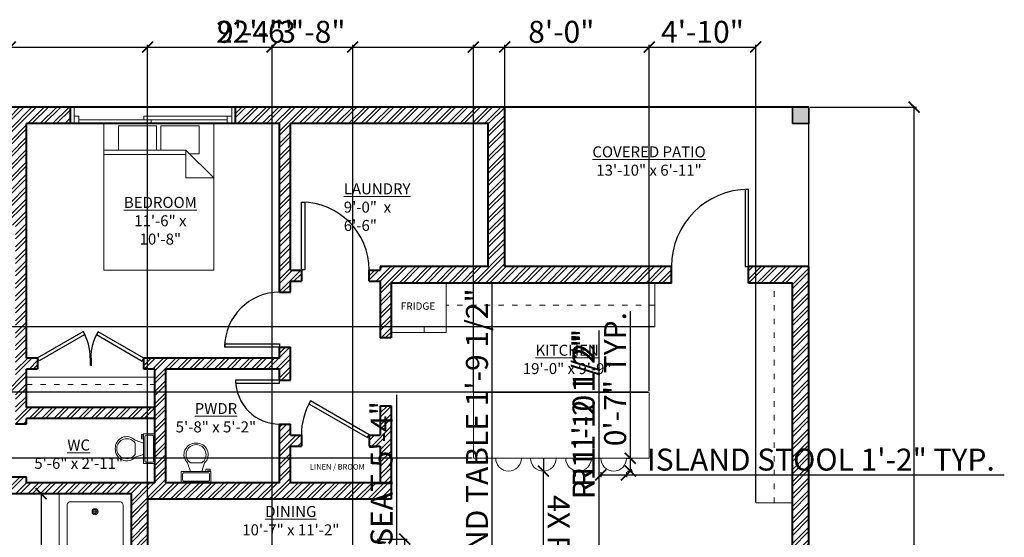
# Model space of a CAD drawing. Units: inches. Extents: x 982 to 1904, y 735 to 1463.
# Tile 7 of 7: x 1301 to 1838, y 1160 to 1443. Entities that reach past the tile are written whole.
import ezdxf

# ---------------------------------------------------------------- set-up
doc = ezdxf.new("R2010")
doc.units = ezdxf.units.IN
doc.linetypes.add('ACAD_ISO03W100', pattern=[30, 12, -18])
for name, color, linetype, lineweight in [('A-ANNO-TEXT', 7, 'Continuous', 18), ('A-AREA-IDEN', 7, 'Continuous', 18), ('A-COLS', 7, 'Continuous', 35), ('A-EQPM', 8, 'Continuous', 18), ('A-FLOR', 7, 'Continuous', 25), ('A-FLOR-CASE', 8, 'Continuous', 20), ('A-FLOR-CASE-HIDN', 8, 'ACAD_ISO03W100', 13), ('A-FLOR-FIXT', 70, 'Continuous', 20), ('Dimensions', 9, 'Continuous', 18), ('Doors', 130, 'Continuous', 25), ('Furniture', 31, 'Continuous', 18), ('Wall Hatch', 23, 'Continuous', 13), ('Walls', 151, 'Continuous', 40), ('Windows', 111, 'Continuous', 18)]:
    doc.layers.add(name, color=color, linetype=linetype, lineweight=lineweight)
doc.layers.add('A-COLS-PATT', color=251, linetype='Continuous', lineweight=13, true_color=0x636466)
doc.styles.get("Standard").update_dxf_attribs({"font": 'arial.ttf'})
doc.dimstyles.new('ISO-25', dxfattribs={"dimtxt": 12, "dimasz": 6, "dimexe": 1.25, "dimexo": 0.625, "dimtad": 1, "dimlunit": 3, "dimtxsty": 'Standard', "dimblk": 'ARCHTICK', "dimcen": 2.5, "dimadec": 0, "dimazin": 0, "dimtfac": 1, "dimtmove": 0, "dimatfit": 3, "dimfxl": 1, "dimarcsym": 0})

# ---------------------------------------------------------------- blocks, each defined once
blk = doc.blocks.new('*U7')
for p, q in [((9.5, -6), (9.5, -2)), ((-10, -8.5), (-8, -8.5)), ((-10, -9.5), (-10, -8.5)), ((-7, -9.5), (-10, -9.5)), ((-8, -8.5), (-8, -8)), ((-7, -8), (-7, -9.5)), ((-4, -8), (-6, -14)), ((4, -8), (6, -14)), ((4, -14), (-4, -14))]:
    blk.add_line(p, q)
blk.add_lwpolyline([(10.5, -8), (10.5, 0), (-10.5, 0), (-10.5, -8)], close=True)
for points in [[(-9.5, -2), (-9.5, -6)], [(8.5, -1), (-8.5, -1)], [(-8.5, -7), (8.5, -7)]]:
    blk.add_lwpolyline(points)
for centre, radius, start, end in [((-8.625, -1.875), 0.8839, 81.8699, 188.1301), ((-8.625, -6.125), 0.8839, 171.869898, 278.1301), ((8.625, -1.875), 0.8839, 351.8699, 98.1301), ((8.625, -6.125), 0.8839, 261.8699, 8.1301), ((-0.4772, -19.9188), 8.0953, 133.01722, 273.38), ((0.0374, -19.8731), 7.127, 124.50543, 269.7), ((-0.0373, -19.8731), 7.127, 270.3, 55.4946), ((0.4773, -19.9188), 8.0953, 266.62, 46.9828)]:
    blk.add_arc(centre, radius, start, end)
blk = doc.blocks.new('*U11')
for p, q in [((0, 0), (0, -100)), ((900, 0), (900, -100))]:
    blk.add_line(p, q)
blk.add_lwpolyline([(0, 0), (0, 900), (43.75, 900), (43.75, 0)], close=True)
blk.add_arc((0, 0), 900, 0, 90)
blk = doc.blocks.new('*U12')
for p, q in [((0, 0), (0, -100)), ((-1000, 0), (-1000, -100))]:
    blk.add_line(p, q)
blk.add_lwpolyline([(0, 0), (0, 1000), (-43.75, 1000), (-43.75, 0)], close=True)
blk.add_arc((0, 0), 1000, 90, 180)
blk = doc.blocks.new('*U13')
for p, q in [((0, 0), (0, -100)), ((-900, 0), (-900, -100))]:
    blk.add_line(p, q)
blk.add_lwpolyline([(0, 0), (-779, 450), (-801, 412), (-22, -38)], close=True)
blk.add_arc((0, 0), 900, 150, 180)
blk = doc.blocks.new('*U14')
for p, q in [((0, 0), (0, -100)), ((750, 0), (750, -100))]:
    blk.add_line(p, q)
blk.add_lwpolyline([(0, 0), (0, 750), (43.75, 750), (43.75, 0)], close=True)
blk.add_arc((0, 0), 750, 0, 90)
blk = doc.blocks.new('*U15')
for p, q in [((-600, 0), (-600, -100)), ((0, 0), (0, -100))]:
    blk.add_line(p, q)
blk.add_lwpolyline([(0, 0), (0, 600), (-43.75, 600), (-43.75, 0)], close=True)
blk.add_arc((0, 0), 600, 90, 180)
blk = doc.blocks.new('Bed - Queen')
for p, q in [((0, -80.00003), (0, 0)), ((0, 0), (59.99999, 0)), ((59.99999, 0), (59.99999, -80.00003)), ((7.99999, -1.2), (28.79998, -1.2)), ((7.99999, -14.4), (7.99999, -1.2)), ((28.79998, -1.2), (28.79998, -14.4)), ((31.19999, -1.2), (51.99999, -1.2)), ((31.19999, -14.4), (31.19999, -1.2)), ((51.99999, -1.2), (51.99999, -16.4)), ((0, -14.4), (44.8, -14.4)), ((59.99999, -29.6), (44.8, -14.4)), ((44.8, -14.4), (44.8, -29.6)), ((44.8, -16.8), (0, -16.8)), ((51.99999, -16.4), (46.79936, -16.4)), ((44.8, -29.6), (59.99999, -29.6)), ((59.99999, -80.00003), (0, -80.00003))]:
    blk.add_line(p, q)
blk = doc.blocks.new('*U17')
for p, q in [((0, 0), (0, -100)), ((700, 0), (700, -100))]:
    blk.add_line(p, q)
blk.add_lwpolyline([(0, 0), (606, 350), (628, 312), (22, -38)], close=True)
blk.add_arc((0, 0), 700, 0, 30)
blk = doc.blocks.new('Bath Tub - 26 x 60 in.')
for p, q in [((8, -18), (10, -18)), ((9, -17), (9, -19))]:
    blk.add_line(p, q)
blk.add_lwpolyline([(0, -36), (0, 0), (60, 0), (60, -36)], close=True)
for points in [[(6, -4), (42, -4)], [(4, -30), (4, -6)], [(42, -32), (6, -32)]]:
    blk.add_lwpolyline(points)
for radius in [1.5, 1]:
    blk.add_circle((9, -18), radius)
for centre, radius, start, end in [((5.75, -5.75), 1.77, 81.8699, 188.1301), ((42, -18), 14, 270, 90), ((5.75, -30.25), 1.77, 171.8699, 278.1301)]:
    blk.add_arc(centre, radius, start, end)
blk = doc.blocks.new('_ArchTick')
at = {"color": 0, "linetype": 'ByBlock', "const_width": 0.15}
blk.add_lwpolyline([(-0.5, -0.5), (0.5, 0.5)], dxfattribs=at)
blk = doc.blocks.new('*D23')
at = {"layer": 'Defpoints', "color": 0, "transparency": 16777216}
for p in [(1731.5, 1394.99), (1788.92, 1394.99), (1732.75, 812.49)]:
    blk.add_point(p, dxfattribs=at)
at = {"layer": 'Dimensions', "color": 0, "lineweight": -2, "transparency": 16777216}
for p, q in [((1732.12, 1394.99), (1790.17, 1394.99)), ((1788.92, 812.49), (1788.92, 1394.99)), ((1733.37, 812.49), (1790.17, 812.49))]:
    blk.add_line(p, q, dxfattribs=at)
at = {"layer": 'Dimensions', "color": 0, "lineweight": -2, "transparency": 16777216, "xscale": 6, "yscale": 6, "zscale": 6}
for p, rotation in [((1788.92, 1394.99), 90), ((1788.92, 812.49), 270)]:
    blk.add_blockref('_ArchTick', p, dxfattribs=dict(at, rotation=rotation))
at = {"layer": 'Dimensions', "color": 0, "transparency": 16777216, "insert": (1782.16, 1103.74), "char_height": 12, "attachment_point": 5, "rotation": 90}
blk.add_mtext('48\'-6.5"', dxfattribs=at)
blk = doc.blocks.new('ISLAND-STOOL-14')
blk.add_arc((7, 7), 7, 180, 0)
blk = doc.blocks.new('*D30')
at = {"layer": 'Defpoints', "color": 0, "transparency": 16777216}
for p in [(1617.95, 1196.33), (1631.95, 1196.33), (1631.95, 1194.23)]:
    blk.add_point(p, dxfattribs=at)
at = {"layer": 'Dimensions', "color": 0, "lineweight": -2, "transparency": 16777216}
for p, q in [((1617.95, 1195.7), (1617.95, 1192.98)), ((1617.95, 1194.23), (1631.95, 1194.23)), ((1631.95, 1195.7), (1631.95, 1192.98)), ((1631.95, 1194.23), (1838.17, 1194.23))]:
    blk.add_line(p, q, dxfattribs=at)
at = {"layer": 'Dimensions', "color": 0, "lineweight": -2, "transparency": 16777216, "xscale": 6, "yscale": 6, "zscale": 6, "rotation": 180}
blk.add_blockref('_ArchTick', (1617.95, 1194.23), dxfattribs=at)
at = {"layer": 'Dimensions', "color": 0, "lineweight": -2, "transparency": 16777216, "xscale": 6, "yscale": 6, "zscale": 6}
blk.add_blockref('_ArchTick', (1631.95, 1194.23), dxfattribs=at)
at = {"layer": 'Dimensions', "color": 0, "transparency": 16777216, "insert": (1738.06, 1201.06), "char_height": 12, "attachment_point": 5}
blk.add_mtext('ISLAND STOOL 1\'-2" TYP.', dxfattribs=at)
blk = doc.blocks.new('*D31')
at = {"layer": 'Defpoints', "color": 0, "transparency": 16777216}
for p in [(1631.95, 1203.33), (1634.05, 1203.33), (1631.95, 1196.33)]:
    blk.add_point(p, dxfattribs=at)
at = {"layer": 'Dimensions', "color": 0, "lineweight": -2, "transparency": 16777216}
for p, q in [((1634.05, 1203.33), (1634.05, 1283.72)), ((1632.57, 1203.33), (1635.3, 1203.33)), ((1634.05, 1196.33), (1634.05, 1203.33)), ((1632.57, 1196.33), (1635.3, 1196.33))]:
    blk.add_line(p, q, dxfattribs=at)
at = {"layer": 'Dimensions', "color": 0, "lineweight": -2, "transparency": 16777216, "xscale": 6, "yscale": 6, "zscale": 6}
for p, rotation in [((1634.05, 1203.33), 90), ((1634.05, 1196.33), 270)]:
    blk.add_blockref('_ArchTick', p, dxfattribs=dict(at, rotation=rotation))
at = {"layer": 'Dimensions', "color": 0, "transparency": 16777216, "insert": (1627.29, 1246.53), "char_height": 12, "attachment_point": 5, "rotation": 90}
blk.add_mtext('0\'-7" TYP.', dxfattribs=at)
blk = doc.blocks.new('*D41')
at = {"layer": 'Defpoints', "color": 0, "transparency": 16777216}
for p in [(1495.17, 1159.23), (1510.97, 1159.23), (1495.17, 1095.57)]:
    blk.add_point(p, dxfattribs=at)
at = {"layer": 'Dimensions', "color": 0, "lineweight": -2, "transparency": 16777216}
for p, q in [((1495.79, 1159.23), (1512.22, 1159.23)), ((1510.97, 1095.57), (1510.97, 1159.23)), ((1495.79, 1095.57), (1512.22, 1095.57))]:
    blk.add_line(p, q, dxfattribs=at)
at = {"layer": 'Dimensions', "color": 0, "lineweight": -2, "transparency": 16777216, "xscale": 6, "yscale": 6, "zscale": 6}
for p, rotation in [((1510.97, 1159.23), 90), ((1510.97, 1095.57), 270)]:
    blk.add_blockref('_ArchTick', p, dxfattribs=dict(at, rotation=rotation))
at = {"layer": 'Dimensions', "color": 0, "transparency": 16777216, "insert": (1504.14, 1127.4), "char_height": 12, "attachment_point": 5, "rotation": 90}
blk.add_mtext('5\'-3 1/2"', dxfattribs=at)
blk = doc.blocks.new('*D44')
at = {"layer": 'Defpoints', "color": 0, "transparency": 16777216}
for p in [(1506.61, 1106.1), (1516.2, 1106.1), (1516.2, 1042.21)]:
    blk.add_point(p, dxfattribs=at)
at = {"layer": 'Dimensions', "color": 0, "lineweight": -2, "transparency": 16777216}
for p, q in [((1506.61, 1106.1), (1506.61, 1237.89)), ((1515.57, 1106.1), (1505.36, 1106.1)), ((1506.61, 1042.21), (1506.61, 1106.1)), ((1515.57, 1042.21), (1505.36, 1042.21))]:
    blk.add_line(p, q, dxfattribs=at)
at = {"layer": 'Dimensions', "color": 0, "lineweight": -2, "transparency": 16777216, "xscale": 6, "yscale": 6, "zscale": 6}
for p, rotation in [((1506.61, 1106.1), 90), ((1506.61, 1042.21), 270)]:
    blk.add_blockref('_ArchTick', p, dxfattribs=dict(at, rotation=rotation))
at = {"layer": 'Dimensions', "color": 0, "transparency": 16777216, "insert": (1499.78, 1175), "char_height": 12, "attachment_point": 5, "rotation": 90}
blk.add_mtext('LOVESEAT 5\'-4"', dxfattribs=at)
blk = doc.blocks.new('*D48')
at = {"layer": 'Defpoints', "color": 0, "transparency": 16777216}
for p in [(1555.46, 1134.17), (1558.68, 1134.17), (1555.46, 1112.72)]:
    blk.add_point(p, dxfattribs=at)
at = {"layer": 'Dimensions', "color": 0, "lineweight": -2, "transparency": 16777216}
for p, q in [((1558.68, 1134.17), (1558.68, 1298.47)), ((1556.09, 1134.17), (1559.93, 1134.17)), ((1558.68, 1112.72), (1558.68, 1134.17)), ((1556.09, 1112.72), (1559.93, 1112.72))]:
    blk.add_line(p, q, dxfattribs=at)
at = {"layer": 'Dimensions', "color": 0, "lineweight": -2, "transparency": 16777216, "xscale": 6, "yscale": 6, "zscale": 6}
for p, rotation in [((1558.68, 1134.17), 90), ((1558.68, 1112.72), 270)]:
    blk.add_blockref('_ArchTick', p, dxfattribs=dict(at, rotation=rotation))
at = {"layer": 'Dimensions', "color": 0, "transparency": 16777216, "insert": (1551.85, 1219.32), "char_height": 12, "attachment_point": 5, "rotation": 90}
blk.add_mtext('END TABLE 1\'-9 1/2"', dxfattribs=at)
blk = doc.blocks.new('*D52')
at = {"layer": 'Defpoints', "color": 0, "transparency": 16777216}
for p in [(1322.2, 1183.99), (1312.37, 1118.49), (1322.2, 1118.49)]:
    blk.add_point(p, dxfattribs=at)
at = {"layer": 'Dimensions', "color": 0, "lineweight": -2, "transparency": 16777216}
for p, q in [((1321.57, 1183.99), (1311.12, 1183.99)), ((1312.37, 1183.99), (1312.37, 1118.49)), ((1321.57, 1118.49), (1311.12, 1118.49)), ((1312.37, 1118.49), (1312.37, 969.02))]:
    blk.add_line(p, q, dxfattribs=at)
at = {"layer": 'Dimensions', "color": 0, "lineweight": -2, "transparency": 16777216, "xscale": 6, "yscale": 6, "zscale": 6}
for p, rotation in [((1312.37, 1183.99), 90), ((1312.37, 1118.49), 270)]:
    blk.add_blockref('_ArchTick', p, dxfattribs=dict(at, rotation=rotation))
at = {"layer": 'Dimensions', "color": 0, "transparency": 16777216, "insert": (1305.54, 1040.75), "char_height": 12, "attachment_point": 5, "rotation": 90}
blk.add_mtext('BATHTUB 5\'-5 1/2"', dxfattribs=at)
blk = doc.blocks.new('*D60')
at = {"layer": 'Defpoints', "color": 0, "transparency": 16777216}
for p in [(1565.5, 1427.79), (1295.5, 1394.99), (1565.5, 1394.99)]:
    blk.add_point(p, dxfattribs=at)
at = {"layer": 'Dimensions', "color": 0, "lineweight": -2, "transparency": 16777216}
for p, q in [((1295.5, 1395.62), (1295.5, 1429.04)), ((1295.5, 1427.79), (1565.5, 1427.79)), ((1565.5, 1395.62), (1565.5, 1429.04))]:
    blk.add_line(p, q, dxfattribs=at)
at = {"layer": 'Dimensions', "color": 0, "lineweight": -2, "transparency": 16777216, "xscale": 6, "yscale": 6, "zscale": 6, "rotation": 180}
blk.add_blockref('_ArchTick', (1295.5, 1427.79), dxfattribs=at)
at = {"layer": 'Dimensions', "color": 0, "lineweight": -2, "transparency": 16777216, "xscale": 6, "yscale": 6, "zscale": 6}
blk.add_blockref('_ArchTick', (1565.5, 1427.79), dxfattribs=at)
at = {"layer": 'Dimensions', "color": 0, "transparency": 16777216, "insert": (1430.5, 1434.54), "char_height": 12, "attachment_point": 5}
blk.add_mtext('22\'-6"', dxfattribs=at)
blk = doc.blocks.new('*D64')
at = {"layer": 'Defpoints', "color": 0, "transparency": 16777216}
for p in [(1482.5, 1427.79), (1370.5, 841.99), (1482.5, 841.99)]:
    blk.add_point(p, dxfattribs=at)
at = {"layer": 'Dimensions', "color": 0, "lineweight": -2, "transparency": 16777216}
for p, q in [((1370.5, 842.62), (1370.5, 1429.04)), ((1370.5, 1427.79), (1482.5, 1427.79)), ((1482.5, 842.62), (1482.5, 1429.04))]:
    blk.add_line(p, q, dxfattribs=at)
at = {"layer": 'Dimensions', "color": 0, "lineweight": -2, "transparency": 16777216, "xscale": 6, "yscale": 6, "zscale": 6, "rotation": 180}
blk.add_blockref('_ArchTick', (1370.5, 1427.79), dxfattribs=at)
at = {"layer": 'Dimensions', "color": 0, "lineweight": -2, "transparency": 16777216, "xscale": 6, "yscale": 6, "zscale": 6}
blk.add_blockref('_ArchTick', (1482.5, 1427.79), dxfattribs=at)
at = {"layer": 'Dimensions', "color": 0, "transparency": 16777216, "insert": (1426.5, 1434.54), "char_height": 12, "attachment_point": 5}
blk.add_mtext('9\'-4"', dxfattribs=at)
blk = doc.blocks.new('*D66')
at = {"layer": 'Defpoints', "color": 0, "transparency": 16777216}
for p in [(1482.5, 1427.79), (1438.5, 1043.01), (1482.5, 1043.03)]:
    blk.add_point(p, dxfattribs=at)
at = {"layer": 'Dimensions', "color": 0, "lineweight": -2, "transparency": 16777216}
for p, q in [((1438.5, 1043.64), (1438.5, 1429.04)), ((1438.5, 1427.79), (1482.5, 1427.79)), ((1482.5, 1043.65), (1482.5, 1429.04))]:
    blk.add_line(p, q, dxfattribs=at)
at = {"layer": 'Dimensions', "color": 0, "lineweight": -2, "transparency": 16777216, "xscale": 6, "yscale": 6, "zscale": 6, "rotation": 180}
blk.add_blockref('_ArchTick', (1438.5, 1427.79), dxfattribs=at)
at = {"layer": 'Dimensions', "color": 0, "lineweight": -2, "transparency": 16777216, "xscale": 6, "yscale": 6, "zscale": 6}
blk.add_blockref('_ArchTick', (1482.5, 1427.79), dxfattribs=at)
at = {"layer": 'Dimensions', "color": 0, "transparency": 16777216, "insert": (1460.5, 1434.55), "char_height": 12, "attachment_point": 5}
blk.add_mtext('3\'-8"', dxfattribs=at)
blk = doc.blocks.new('*D67')
at = {"layer": 'Defpoints', "color": 0, "transparency": 16777216}
for p in [(1644.35, 1427.79), (1548.35, 1239.33), (1644.35, 1239.33)]:
    blk.add_point(p, dxfattribs=at)
at = {"layer": 'Dimensions', "color": 0, "lineweight": -2, "transparency": 16777216}
for p, q in [((1548.35, 1239.95), (1548.35, 1429.04)), ((1548.35, 1427.79), (1644.35, 1427.79)), ((1644.35, 1239.95), (1644.35, 1429.04))]:
    blk.add_line(p, q, dxfattribs=at)
at = {"layer": 'Dimensions', "color": 0, "lineweight": -2, "transparency": 16777216, "xscale": 6, "yscale": 6, "zscale": 6, "rotation": 180}
blk.add_blockref('_ArchTick', (1548.35, 1427.79), dxfattribs=at)
at = {"layer": 'Dimensions', "color": 0, "lineweight": -2, "transparency": 16777216, "xscale": 6, "yscale": 6, "zscale": 6}
blk.add_blockref('_ArchTick', (1644.35, 1427.79), dxfattribs=at)
at = {"layer": 'Dimensions', "color": 0, "transparency": 16777216, "insert": (1596.35, 1434.54), "char_height": 12, "attachment_point": 5}
blk.add_mtext('8\'-0"', dxfattribs=at)
blk = doc.blocks.new('*D68')
at = {"layer": 'Defpoints', "color": 0, "transparency": 16777216}
for p in [(1548.35, 1239.33), (1123.7, 1203.33), (1548.35, 1203.33)]:
    blk.add_point(p, dxfattribs=at)
at = {"layer": 'Dimensions', "color": 0, "lineweight": -2, "transparency": 16777216}
for p, q in [((1547.73, 1239.33), (1122.45, 1239.33)), ((1123.7, 1239.33), (1123.7, 1203.33)), ((1547.73, 1203.33), (1122.45, 1203.33))]:
    blk.add_line(p, q, dxfattribs=at)
at = {"layer": 'Dimensions', "color": 0, "lineweight": -2, "transparency": 16777216, "xscale": 6, "yscale": 6, "zscale": 6}
for p, rotation in [((1123.7, 1239.33), 90), ((1123.7, 1203.33), 270)]:
    blk.add_blockref('_ArchTick', p, dxfattribs=dict(at, rotation=rotation))
at = {"layer": 'Dimensions', "color": 0, "transparency": 16777216, "insert": (1116.94, 1221.33), "char_height": 12, "attachment_point": 5, "rotation": 90}
blk.add_mtext('3\'-0"', dxfattribs=at)
blk = doc.blocks.new('*D69')
at = {"layer": 'Defpoints', "color": 0, "transparency": 16777216}
for p in [(1123.7, 1274.99), (1647.5, 1274.99), (1644.35, 1239.33)]:
    blk.add_point(p, dxfattribs=at)
at = {"layer": 'Dimensions', "color": 0, "lineweight": -2, "transparency": 16777216}
for p, q in [((1123.7, 1274.99), (1123.7, 1351.63)), ((1646.87, 1274.99), (1122.45, 1274.99)), ((1123.7, 1239.33), (1123.7, 1274.99)), ((1643.73, 1239.33), (1122.45, 1239.33))]:
    blk.add_line(p, q, dxfattribs=at)
at = {"layer": 'Dimensions', "color": 0, "lineweight": -2, "transparency": 16777216, "xscale": 6, "yscale": 6, "zscale": 6}
for p, rotation in [((1123.7, 1274.99), 90), ((1123.7, 1239.33), 270)]:
    blk.add_blockref('_ArchTick', p, dxfattribs=dict(at, rotation=rotation))
at = {"layer": 'Dimensions', "color": 0, "transparency": 16777216, "insert": (1116.87, 1316.31), "char_height": 12, "attachment_point": 5, "rotation": 90}
blk.add_mtext('2\'-11 1/2"', dxfattribs=at)
blk = doc.blocks.new('*D70')
at = {"layer": 'Defpoints', "color": 0, "transparency": 16777216}
for p in [(1702.5, 1427.79), (1644.35, 1239.33), (1702.5, 1178.99)]:
    blk.add_point(p, dxfattribs=at)
at = {"layer": 'Dimensions', "color": 0, "lineweight": -2, "transparency": 16777216}
for p, q in [((1644.35, 1239.95), (1644.35, 1429.04)), ((1644.35, 1427.79), (1702.5, 1427.79)), ((1702.5, 1179.62), (1702.5, 1429.04))]:
    blk.add_line(p, q, dxfattribs=at)
at = {"layer": 'Dimensions', "color": 0, "lineweight": -2, "transparency": 16777216, "xscale": 6, "yscale": 6, "zscale": 6, "rotation": 180}
blk.add_blockref('_ArchTick', (1644.35, 1427.79), dxfattribs=at)
at = {"layer": 'Dimensions', "color": 0, "lineweight": -2, "transparency": 16777216, "xscale": 6, "yscale": 6, "zscale": 6}
blk.add_blockref('_ArchTick', (1702.5, 1427.79), dxfattribs=at)
at = {"layer": 'Dimensions', "color": 0, "transparency": 16777216, "insert": (1673.42, 1434.54), "char_height": 12, "attachment_point": 5}
blk.add_mtext('4\'-10"', dxfattribs=at)
blk = doc.blocks.new('*D73')
at = {"layer": 'Defpoints', "color": 0, "transparency": 16777216}
for p in [(1616.91, 1141.97), (1616.91, 999.48)]:
    blk.add_point(p, dxfattribs=at)
at = {"layer": 'Dimensions', "color": 0, "lineweight": -2, "transparency": 16777216}
for p in [(1616.91, 1273.09), (1616.91, 999.48)]:
    blk.add_line(p, (1616.91, 1141.97), dxfattribs=at)
at = {"layer": 'Dimensions', "color": 0, "lineweight": -2, "transparency": 16777216, "xscale": 6, "yscale": 6, "zscale": 6, "rotation": 269.9998576619989}
blk.add_blockref('_ArchTick', (1616.91, 1141.97), dxfattribs=at)
at = {"layer": 'Dimensions', "color": 0, "transparency": 16777216, "insert": (1610.08, 1227.47), "char_height": 12, "attachment_point": 5, "rotation": 89.9999}
blk.add_mtext('R11\'-10 1/2"', dxfattribs=at)
blk = doc.blocks.new('*D74')
at = {"layer": 'Defpoints', "color": 0, "transparency": 16777216}
for p in [(1616.91, 1149.03), (1616.91, 1014.7)]:
    blk.add_point(p, dxfattribs=at)
at = {"layer": 'Dimensions', "color": 0, "lineweight": -2, "transparency": 16777216}
for p in [(1616.91, 1270.59), (1616.91, 1014.7)]:
    blk.add_line(p, (1616.91, 1149.03), dxfattribs=at)
at = {"layer": 'Dimensions', "color": 0, "lineweight": -2, "transparency": 16777216, "xscale": 6, "yscale": 6, "zscale": 6, "rotation": 269.9998536992126}
blk.add_blockref('_ArchTick', (1616.91, 1149.03), dxfattribs=at)
at = {"layer": 'Dimensions', "color": 0, "transparency": 16777216, "insert": (1610.08, 1229.63), "char_height": 12, "attachment_point": 5, "rotation": 89.9999}
blk.add_mtext('R11\'-2 1/2"', dxfattribs=at)
blk = doc.blocks.new('*D79')
at = {"layer": 'Defpoints', "color": 0, "transparency": 16777216}
for p in [(1586.55, 1203.33), (1586.55, 1196.33)]:
    blk.add_point(p, dxfattribs=at)
at = {"layer": 'Dimensions', "color": 0, "lineweight": -2, "transparency": 16777216}
for p in [(1586.55, 1203.33), (1586.55, 1113.43)]:
    blk.add_line(p, (1586.55, 1196.33), dxfattribs=at)
at = {"layer": 'Dimensions', "color": 0, "lineweight": -2, "transparency": 16777216, "xscale": 6, "yscale": 6, "zscale": 6, "rotation": 90.00372422566393}
blk.add_blockref('_ArchTick', (1586.55, 1196.33), dxfattribs=at)
at = {"layer": 'Dimensions', "color": 0, "transparency": 16777216, "insert": (1593.3, 1148.88), "char_height": 12, "attachment_point": 5, "rotation": 270.0037}
blk.add_mtext('4X R0\'-7"', dxfattribs=at)

msp = doc.modelspace()

# ---------------------------------------------------------------- hatches: boundary and pattern name
at = {"layer": 'A-COLS-PATT'}
h = msp.add_hatch(color=256, dxfattribs=at)
h.dxf.hatch_style = 1
h.paths.add_polyline_path([(1731.496, 1394.991), (1722.496, 1394.991), (1722.496, 1385.991), (1731.496, 1385.991)])
h.paths.add_polyline_path([(1725.019, 843.656), (1721.019, 843.656), (1721.019, 837.656), (1725.019, 837.656)])
h.paths.add_polyline_path([(1734.019, 843.656), (1730.019, 843.656), (1730.019, 837.656), (1734.019, 837.656)])
h.paths.add_polyline_path([(1483.18, 791.991), (1479.18, 791.991), (1479.18, 785.991), (1483.18, 785.991)])
h.paths.add_polyline_path([(1492.18, 791.991), (1488.18, 791.991), (1488.18, 785.991), (1492.18, 785.991)])
h.paths.add_polyline_path([(1364.813, 791.991), (1360.813, 791.991), (1360.813, 785.991), (1364.813, 785.991)])
h.paths.add_polyline_path([(1373.813, 791.991), (1369.813, 791.991), (1369.813, 785.991), (1373.813, 785.991)])
at = {"layer": 'Wall Hatch'}
h = msp.add_hatch(dxfattribs=at)
h.set_pattern_fill('ANSI32', color=256, scale=0.5)
h.paths.add_polyline_path([(1165.496, 1065.991), (1271.496, 1065.991), (1271.496, 1071.991), (1218.496, 1071.991), (1218.496, 1238.491), (1262.496, 1238.491), (1262.496, 1244.491), (1218.496, 1244.491), (1218.496, 1330.491), (1298.496, 1330.491), (1298.496, 1244.491), (1292.496, 1244.491), (1292.496, 1238.491), (1298.496, 1238.491), (1298.496, 1221.991), (1304.496, 1221.991), (1304.496, 1224.991), (1374.496, 1224.991), (1374.496, 1230.991), (1304.496, 1230.991), (1304.496, 1251.991), (1310.496, 1251.991), (1310.496, 1257.991), (1304.496, 1257.991), (1304.496, 1385.991), (1328.496, 1385.991), (1328.496, 1394.991), (1295.496, 1394.991), (1295.496, 1339.491), (1209.496, 1339.491), (1209.496, 1071.991), (1156.496, 1071.991), (1156.496, 893.991), (1171.496, 893.991), (1171.496, 902.991), (1165.496, 902.991)])
h.paths.add_polyline_path([(1273.996, 877.991), (1267.996, 877.991), (1267.996, 902.991), (1252.996, 902.991), (1252.996, 893.991), (1258.996, 893.991), (1258.996, 868.991), (1273.996, 868.991)])
h.paths.add_polyline_path([(1370.496, 1052.991), (1361.496, 1052.991), (1361.496, 1046.991), (1355.496, 1046.991), (1355.496, 1040.991), (1361.496, 1040.991), (1361.496, 877.991), (1355.496, 877.991), (1355.496, 868.991), (1361.496, 868.991), (1361.496, 832.991), (1376.313, 832.991), (1491.496, 832.991), (1491.496, 985.991), (1515.496, 985.991), (1515.496, 994.991), (1482.496, 994.991), (1482.496, 841.991), (1370.496, 841.991)])
h.paths.add_polyline_path([(1319.496, 1088.991), (1325.496, 1088.991), (1325.496, 1094.991), (1319.496, 1094.991), (1319.496, 1112.491), (1361.496, 1112.491), (1361.496, 1094.991), (1355.496, 1094.991), (1355.496, 1088.991), (1361.496, 1088.991), (1361.496, 1082.991), (1370.496, 1082.991), (1370.496, 1180.991), (1503.496, 1180.991), (1503.496, 1231.991), (1497.496, 1231.991), (1497.496, 1215.991), (1491.496, 1215.991), (1491.496, 1209.991), (1497.496, 1209.991), (1497.496, 1189.991), (1448.496, 1189.991), (1448.496, 1209.991), (1454.496, 1209.991), (1454.496, 1215.991), (1448.496, 1215.991), (1448.496, 1221.991), (1442.496, 1221.991), (1442.496, 1189.991), (1380.496, 1189.991), (1380.496, 1251.991), (1442.496, 1251.991), (1442.496, 1245.991), (1448.496, 1245.991), (1448.496, 1263.991), (1442.496, 1263.991), (1442.496, 1257.991), (1368.496, 1257.991), (1368.496, 1251.991), (1374.496, 1251.991), (1374.496, 1189.991), (1304.496, 1189.991), (1304.496, 1192.991), (1295.496, 1192.991), (1295.496, 1183.991), (1361.496, 1183.991), (1361.496, 1118.491), (1313.496, 1118.491), (1313.496, 1071.991), (1301.496, 1071.991), (1301.496, 1065.991), (1313.496, 1065.991), (1313.496, 1040.991), (1325.496, 1040.991), (1325.496, 1046.991), (1319.496, 1046.991)])
h.paths.add_polyline_path([(1565.496, 1394.991), (1418.496, 1394.991), (1418.496, 1385.991), (1442.496, 1385.991), (1442.496, 1293.991), (1448.496, 1293.991), (1448.496, 1299.991), (1454.496, 1299.991), (1454.496, 1305.991), (1448.496, 1305.991), (1448.496, 1385.991), (1556.496, 1385.991), (1556.496, 1307.991), (1497.496, 1307.991), (1497.496, 1305.991), (1491.496, 1305.991), (1491.496, 1299.991), (1497.496, 1299.991), (1497.496, 1268.991), (1503.496, 1268.991), (1503.496, 1298.991), (1656.496, 1298.991), (1656.496, 1307.991), (1565.496, 1307.991)])
h.paths.add_polyline_path([(1731.496, 1307.991), (1698.496, 1307.991), (1698.496, 1298.991), (1722.496, 1298.991), (1722.496, 1033.991), (1731.496, 1033.991)])
h.paths.add_polyline_path([(1731.496, 997.991), (1722.496, 997.991), (1722.496, 994.991), (1689.496, 994.991), (1689.496, 985.991), (1731.496, 985.991)])

# ---------------------------------------------------------------- linework, layer by layer
at = {"layer": 'A-COLS'}
msp.add_lwpolyline([(1722.496, 1385.991), (1731.496, 1385.991), (1731.496, 1394.991), (1722.496, 1394.991)], close=True, dxfattribs=at)
at = {"layer": 'A-EQPM'}
for p, q in [((1533.496, 1298.991), (1533.496, 1271.991)), ((1521.496, 1274.991), (1521.496, 1271.991)), ((1533.496, 1271.991), (1503.496, 1271.991))]:
    msp.add_line(p, q, dxfattribs=at)
at = {"layer": 'A-FLOR'}
msp.add_line((1731.496, 1307.991), (1731.496, 1394.991), dxfattribs=at)
at = {"layer": 'A-FLOR-CASE'}
for p, q in [((1647.496, 1298.991), (1647.496, 1274.991)), ((1702.496, 1178.991), (1702.496, 1298.991)), ((1647.496, 1274.991), (1503.496, 1274.991)), ((1304.496, 1247.688), (1374.496, 1247.688)), ((1644.351, 1239.328), (1548.351, 1239.328)), ((1548.351, 1239.328), (1548.351, 1203.328)), ((1644.351, 1203.328), (1644.351, 1239.328)), ((1548.351, 1203.328), (1644.351, 1203.328)), ((1722.496, 1178.991), (1702.496, 1178.991))]:
    msp.add_line(p, q, dxfattribs=at)
at = {"layer": 'A-FLOR-CASE-HIDN', "ltscale": 0.25}
for p, q in [((1712.496, 1178.991), (1712.496, 1298.991)), ((1647.496, 1286.991), (1533.496, 1286.991)), ((1304.496, 1243.688), (1374.496, 1243.688))]:
    msp.add_line(p, q, dxfattribs=at)
at = {"layer": 'Walls'}
for p, q in [((1731.496, 1394.991), (1295.496, 1394.991)), ((1328.496, 1385.991), (1328.496, 1394.991)), ((1418.496, 1385.991), (1418.496, 1394.991)), ((1565.496, 1307.991), (1565.496, 1394.991)), ((1442.496, 1385.991), (1304.496, 1385.991)), ((1304.496, 1257.991), (1304.496, 1385.991)), ((1442.496, 1293.991), (1442.496, 1385.991)), ((1556.496, 1385.991), (1448.496, 1385.991)), ((1448.496, 1305.991), (1448.496, 1385.991)), ((1556.496, 1307.991), (1556.496, 1385.991)), ((1497.496, 1307.991), (1497.496, 1305.991)), ((1556.496, 1307.991), (1497.496, 1307.991)), ((1656.496, 1307.991), (1565.496, 1307.991)), ((1656.496, 1298.991), (1656.496, 1307.991)), ((1731.496, 1307.991), (1698.496, 1307.991)), ((1698.496, 1298.991), (1698.496, 1307.991)), ((1731.496, 985.991), (1731.496, 1307.991)), ((1448.496, 1305.991), (1454.496, 1305.991)), ((1454.496, 1305.991), (1454.496, 1299.991)), ((1491.496, 1305.991), (1497.496, 1305.991)), ((1491.496, 1299.991), (1491.496, 1305.991)), ((1448.496, 1299.991), (1454.496, 1299.991)), ((1448.496, 1293.991), (1448.496, 1299.991)), ((1491.496, 1299.991), (1497.496, 1299.991)), ((1497.496, 1299.991), (1497.496, 1268.991)), ((1503.496, 1298.991), (1503.496, 1268.991)), ((1656.496, 1298.991), (1503.496, 1298.991)), ((1722.496, 1298.991), (1698.496, 1298.991)), ((1722.496, 994.991), (1722.496, 1298.991)), ((1442.496, 1293.991), (1448.496, 1293.991)), ((1503.496, 1268.991), (1497.496, 1268.991)), ((1442.496, 1263.991), (1448.496, 1263.991)), ((1442.496, 1257.991), (1442.496, 1263.991)), ((1448.496, 1245.991), (1448.496, 1263.991)), ((1310.496, 1257.991), (1304.496, 1257.991)), ((1310.496, 1257.991), (1310.496, 1251.991)), ((1442.496, 1257.991), (1368.496, 1257.991)), ((1368.496, 1251.991), (1368.496, 1257.991)), ((1310.496, 1251.991), (1304.496, 1251.991)), ((1304.496, 1230.991), (1304.496, 1251.991)), ((1374.496, 1251.991), (1368.496, 1251.991)), ((1374.496, 1189.991), (1374.496, 1251.991)), ((1442.496, 1251.991), (1380.496, 1251.991)), ((1380.496, 1189.991), (1380.496, 1251.991)), ((1442.496, 1245.991), (1442.496, 1251.991)), ((1442.496, 1245.991), (1448.496, 1245.991)), ((1374.496, 1230.991), (1304.496, 1230.991)), ((1497.496, 1231.991), (1503.496, 1231.991)), ((1497.496, 1231.991), (1497.496, 1215.991)), ((1503.496, 1231.991), (1503.496, 1180.991)), ((1304.496, 1221.991), (1298.496, 1221.991)), ((1374.496, 1224.991), (1304.496, 1224.991)), ((1304.496, 1221.991), (1304.496, 1224.991)), ((1442.496, 1189.991), (1442.496, 1221.991)), ((1442.496, 1221.991), (1448.496, 1221.991)), ((1448.496, 1215.991), (1448.496, 1221.991)), ((1448.496, 1215.991), (1454.496, 1215.991)), ((1454.496, 1215.991), (1454.496, 1209.991)), ((1491.496, 1215.991), (1497.496, 1215.991)), ((1491.496, 1215.991), (1491.496, 1209.991)), ((1448.496, 1189.991), (1448.496, 1209.991)), ((1448.496, 1209.991), (1454.496, 1209.991)), ((1491.496, 1209.991), (1497.496, 1209.991)), ((1497.496, 1209.991), (1497.496, 1189.991)), ((1304.496, 1192.991), (1295.496, 1192.991)), ((1304.496, 1189.991), (1304.496, 1192.991)), ((1374.496, 1189.991), (1304.496, 1189.991)), ((1442.496, 1189.991), (1380.496, 1189.991)), ((1497.496, 1189.991), (1448.496, 1189.991)), ((1361.496, 1183.991), (1295.496, 1183.991)), ((1361.496, 1183.991), (1361.496, 1118.491)), ((1503.496, 1180.991), (1370.496, 1180.991)), ((1370.496, 1180.991), (1370.496, 1082.991))]:
    msp.add_line(p, q, dxfattribs=at)
at = {"layer": 'Windows'}
for p, q in [((1330.496, 1385.991), (1330.496, 1394.991)), ((1416.496, 1385.991), (1416.496, 1394.991)), ((1332.996, 1389.991), (1330.496, 1389.991)), ((1413.996, 1387.991), (1332.996, 1387.991)), ((1368.496, 1387.991), (1368.496, 1389.991)), ((1416.496, 1389.991), (1368.496, 1389.991)), ((1372.496, 1385.991), (1372.496, 1387.991))]:
    msp.add_line(p, q, dxfattribs=at)
for points in [[(1330.496, 1385.991), (1332.996, 1385.991), (1332.996, 1389.991), (1330.496, 1389.991)], [(1413.996, 1385.991), (1416.496, 1385.991), (1416.496, 1389.991), (1413.996, 1389.991)]]:
    msp.add_lwpolyline(points, close=True, dxfattribs=at)

# ---------------------------------------------------------------- block references
at = {"layer": 'A-FLOR-FIXT'}
for name, p, xscale, yscale, zscale, rotation in [('*U7', (1374.496, 1208.541), 0.7704630167235674, 0.7704630167235674, 0.7704630167235674, 270), ('*U7', (1396.995, 1189.991), 0.7704630167235677, 0.7704630167235677, 0.7704630167235677, 179.9999999999998), ('Bath Tub - 26 x 60 in.', (1361.496, 1183.991), 1.091666666666662, 1.091666666666662, 1.091666666666662, 270)]:
    msp.add_blockref(name, p, dxfattribs=dict(at, xscale=xscale, yscale=yscale, zscale=zscale, rotation=rotation))
at = {"layer": 'Doors'}
for name, p, xscale, yscale, zscale in [('*U12', (1698.496, 1308.08), 0.0420018003729353, 0.0420018003729353, 0.0420018003729353), ('*U11', (1454.496, 1306.102), 0.0411111111111105, 0.0411111111111105, 0.0411111111111105), ('*U17', (1310.496, 1258.102), 0.0411111111111105, 0.0411111111111105, 0.0411111111111105), ('*U17', (1368.496, 1257.991), -0.0411111111111105, 0.0411111111111105, 0.0411111111111105), ('*U13', (1491.496, 1216.165), 0.0411111111111107, 0.0411111111111107, 0.0411111111111107)]:
    msp.add_blockref(name, p, dxfattribs=dict(at, xscale=xscale, yscale=yscale, zscale=zscale))
at = {"layer": 'Doors', "xscale": 0.0400014610004212, "yscale": 0.0400014610004212, "zscale": 0.0400014610004212, "rotation": 89.99999999999999}
for name, p in [('*U14', (1442.607, 1263.991)), ('*U15', (1442.607, 1245.992))]:
    msp.add_blockref(name, p, dxfattribs=at)
at = {"layer": 'Furniture'}
for name, p in [('Bed - Queen', (1346.613, 1385.991)), ('ISLAND-STOOL-14', (1560.552, 1196.328)), ('ISLAND-STOOL-14', (1579.547, 1196.328)), ('ISLAND-STOOL-14', (1598.747, 1196.328)), ('ISLAND-STOOL-14', (1617.947, 1196.328))]:
    msp.add_blockref(name, p, dxfattribs=at)

# ---------------------------------------------------------------- texts
at = {"layer": 'A-ANNO-TEXT', "attachment_point": 1}
for s, width, insert, char_height in [('{\\fTimes New Roman|b0|i0|c0|p18;FRIDGE}', 30.01819, (1508.712, 1288.385), 4), ('\\pxqc;{\\fTimes New Roman|b0|i0|c0|p18;\\T1.25;LINEN / BROOM}', 39.88823, (1454.122, 1200.161), 3)]:
    msp.add_mtext_dynamic_manual_height_columns(s, width=width, gutter_width=12.5, heights=[0], dxfattribs=dict(at, insert=insert, char_height=char_height))
at = {"layer": 'A-AREA-IDEN', "char_height": 6, "attachment_point": 1}
for s, width, insert in [('\\pxqc;{\\fTimes New Roman|b0|i0|c0|p18;\\LCOVERED PATIO\\P\\l13\'-10" x 6\'-11"}', 97.51841, (1595.484, 1373.589)), ('{\\fTimes New Roman|b0|i0|c0|p18;\\LLAUNDRY\\P\\l9\'-0"  x 6\'-6"}', 44.9592, (1477.636, 1353.413)), ('\\pxqc;{\\fTimes New Roman|b0|i0|c0|p18;\\LBEDROOM\\P\\l11\'-6" x 10\'-8"}', 52.44419, (1351.279, 1345.991)), ('\\pxqc;{\\fTimes New Roman|b0|i0|c0|p18;\\LKITCHEN\\P\\l19\'-0" x 9\'-9"}', 95.90504, (1551.606, 1265.283)), ('\\pxqc;{\\fTimes New Roman|b0|i0|c0|p18;\\LPWDR\\P\\l5\'-8" x 5\'-2"}', 49.70298, (1382.978, 1233.462)), ('\\pxqc;{\\fTimes New Roman|b0|i0|c0|p18;\\LWC\\P\\l5\'-6" x 2\'-11"}', 49.73342, (1308.053, 1213.575)), ('\\pxqc;{\\fTimes New Roman|b0|i0|c0|p18;\\LDINING\\P\\l10\'-7" x 11\'-2"}', 53.79244, (1421.822, 1177.278))]:
    msp.add_mtext_dynamic_manual_height_columns(s, width=width, gutter_width=12.5, heights=[0], dxfattribs=dict(at, insert=insert))

# ---------------------------------------------------------------- dimensions: what is measured, and where the dimension line sits
at = {"layer": 'Dimensions'}
for base, p1, p2, picture, middle in [((1565.496, 1427.791), (1295.496, 1394.991), (1565.496, 1394.991), '*D60', (1430.496, 1434.543)), ((1482.496, 1427.791), (1370.496, 841.991), (1482.496, 841.991), '*D64', (1426.496, 1434.543)), ((1482.496, 1427.791), (1438.496, 1043.012), (1482.496, 1043.025), '*D66', (1460.496, 1434.547)), ((1644.351, 1427.791), (1548.351, 1239.328), (1644.351, 1239.328), '*D67', (1596.351, 1434.543)), ((1702.496, 1427.791), (1644.351, 1239.328), (1702.496, 1178.991), '*D70', (1673.424, 1434.543))]:
    dim = msp.add_linear_dim(base=base, p1=p1, p2=p2, dimstyle='ISO-25', override={"dimdec": 1, "dimlfac": 1, "dimrnd": 0, "dimzin": 1, "dimdsep": 46, "dimlunit": 4, "dimfrac": 2}, dxfattribs=at)
    dim.commit()
    dim.dimension.update_dxf_attribs({"geometry": picture, "text_midpoint": middle})
for base, p1, p2, override, picture, middle in [((1788.915, 1394.991), (1732.746, 812.491), (1731.496, 1394.991), {"dimclrd": 0, "dimclre": 0, "dimclrt": 0}, '*D23', (1782.164, 1103.741)), ((1123.696, 1274.991), (1644.351, 1239.328), (1647.496, 1274.991), {"dimdec": 1, "dimlfac": 1, "dimrnd": 0, "dimzin": 1, "dimdsep": 46, "dimlunit": 4, "dimfrac": 2}, '*D69', (1116.867, 1316.31)), ((1123.696, 1203.328), (1548.351, 1239.328), (1548.351, 1203.328), {"dimdec": 1, "dimlfac": 1, "dimrnd": 0, "dimzin": 1, "dimdsep": 46, "dimlunit": 4, "dimfrac": 2}, '*D68', (1116.94, 1221.328)), ((1510.969, 1159.23), (1495.169, 1095.569), (1495.169, 1159.23), {"dimdec": 1, "dimlfac": 1, "dimrnd": 0, "dimzin": 1, "dimdsep": 46, "dimlunit": 4, "dimfrac": 2}, '*D41', (1504.135, 1127.4))]:
    dim = msp.add_linear_dim(base=base, p1=p1, p2=p2, angle=90, dimstyle='ISO-25', override=override, dxfattribs=at)
    dim.commit()
    dim.dimension.update_dxf_attribs({"geometry": picture, "text_midpoint": middle})
for base, p1, p2, angle, text, picture, middle in [((1558.678, 1134.173), (1555.46, 1112.72), (1555.46, 1134.173), 90, 'END TABLE <>', '*D48', (1551.848, 1219.322)), ((1634.047, 1203.328), (1631.947, 1196.328), (1631.947, 1203.328), 90, '<> TYP.', '*D31', (1627.295, 1246.526)), ((1506.613, 1106.103), (1516.197, 1042.21), (1516.197, 1106.103), 90, 'LOVESEAT <>', '*D44', (1499.779, 1174.996)), ((1312.371, 1118.491), (1322.196, 1183.991), (1322.196, 1118.491), 270, 'BATHTUB <>', '*D52', (1305.542, 1040.754))]:
    dim = msp.add_linear_dim(base=base, p1=p1, p2=p2, angle=angle, text=text, dimstyle='ISO-25', override={"dimdec": 1, "dimlfac": 1, "dimrnd": 0, "dimzin": 1, "dimdsep": 46, "dimlunit": 4, "dimfrac": 2}, dxfattribs=at)
    dim.commit()
    dim.dimension.update_dxf_attribs({"geometry": picture, "text_midpoint": middle})
for center, mpoint, picture, middle in [((1616.913, 999.478), (1616.913, 1141.974), '*D73', (1616.913, 1227.473)), ((1616.913, 1014.7), (1616.913, 1149.029), '*D74', (1616.913, 1229.626))]:
    dim = msp.add_radius_dim(center=center, mpoint=mpoint, dimstyle='ISO-25', override={"dimdec": 1, "dimlfac": 1, "dimrnd": 0, "dimzin": 1, "dimdsep": 46, "dimlunit": 4, "dimfrac": 2}, dxfattribs=at)
    dim.commit()
    dim.dimension.update_dxf_attribs({"geometry": picture, "text_midpoint": middle, "dimtype": 164})
dim = msp.add_linear_dim(base=(1631.947, 1194.228), p1=(1617.947, 1196.328), p2=(1631.947, 1196.328), text='ISLAND STOOL <> TYP.', dimstyle='ISO-25', override={"dimdec": 1, "dimlfac": 1, "dimrnd": 0, "dimzin": 1, "dimdsep": 46, "dimlunit": 4, "dimfrac": 2}, dxfattribs=at)
dim.commit()
dim.dimension.update_dxf_attribs({"geometry": '*D30', "text_midpoint": (1738.059, 1201.062)})
dim = msp.add_radius_dim(center=(1586.547, 1203.328), mpoint=(1586.547, 1196.328), text='4X <>', dimstyle='ISO-25', override={"dimdec": 1, "dimlfac": 1, "dimrnd": 0, "dimzin": 1, "dimdsep": 46, "dimlunit": 4, "dimfrac": 2}, dxfattribs=at)
dim.commit()
dim.dimension.update_dxf_attribs({"geometry": '*D79', "text_midpoint": (1593.302, 1148.878)})

doc.saveas('drawing.dxf')
